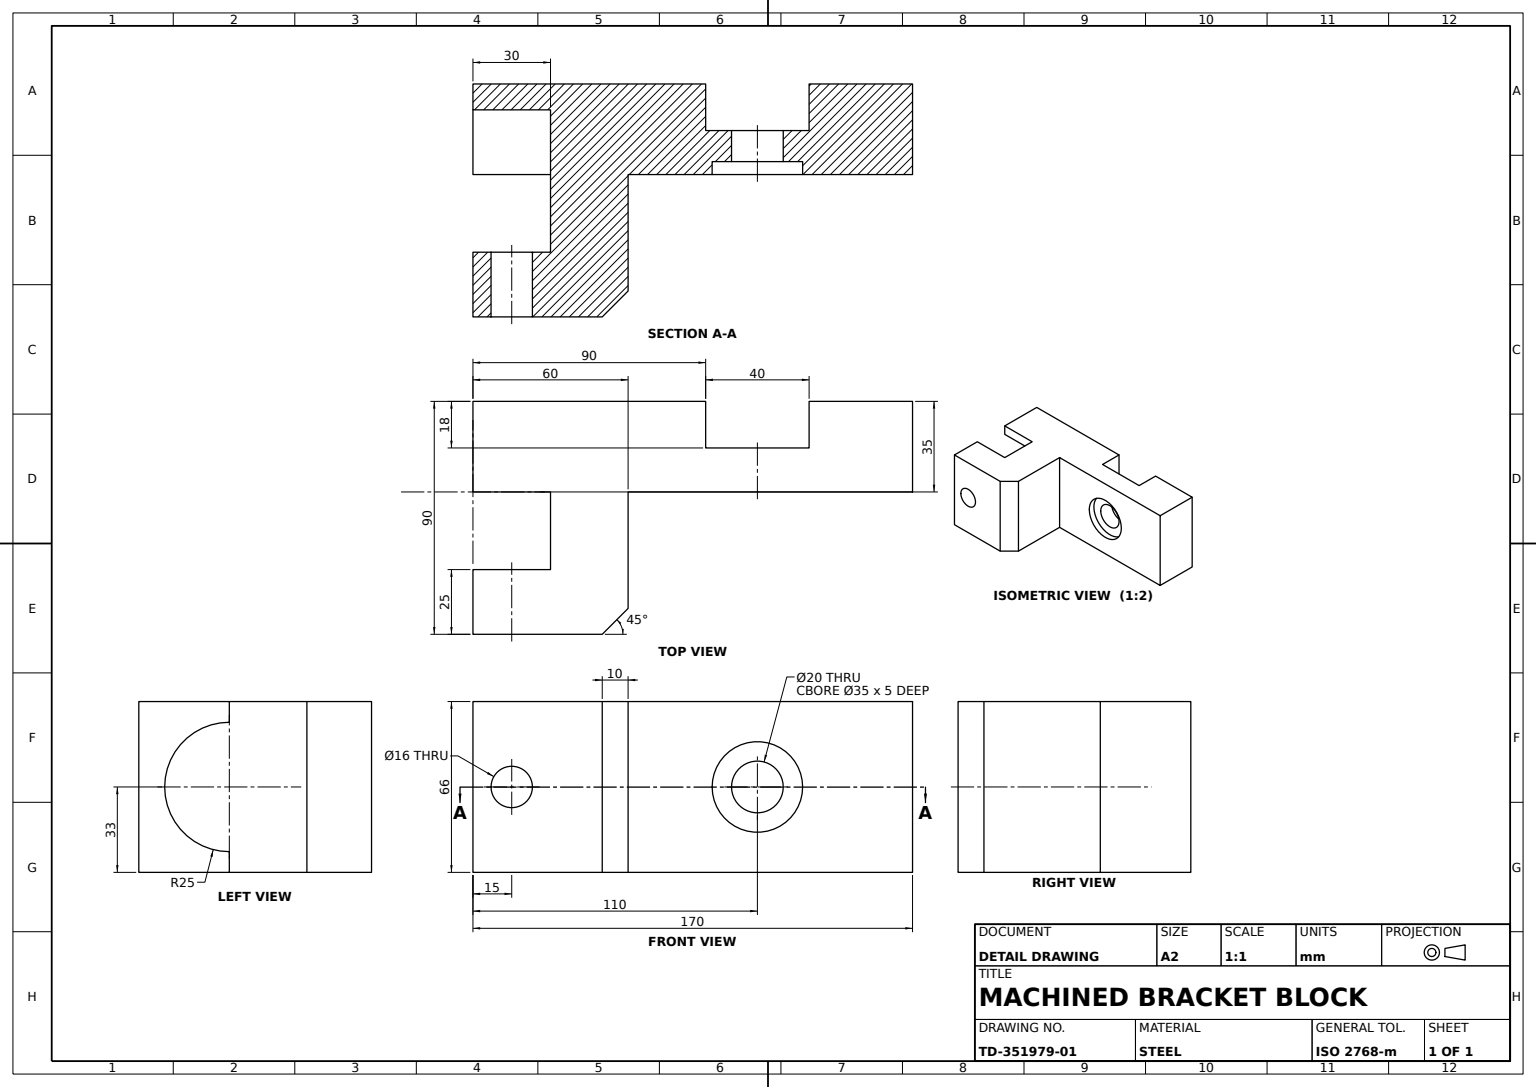
from build123d import *

# Parameters (mm, degrees)
BASE_BLOCK_PROFILE_W    = 170
BASE_BLOCK_PROFILE_H    = 66
BASE_BLOCK_DEPTH        = 35
SLOT_CUT_DEPTH          = 66
COUNTERBORE_35_SKETCH_R = 17.5
COUNTERBORE_35_DEPTH    = 5
HOLE_20_SKETCH_R        = 10
HOLE_20_DEPTH           = 12
ROUNDED_CUT_DEPTH       = 30
SIDE_LUG_DEPTH          = 66
LUG_HOLE_16_SKETCH_R    = 8
LUG_HOLE_16_DEPTH       = 66


with BuildPart() as part:
    # Base Block Profile → Base Block (new body)
    with BuildSketch(Plane.XY):
        with Locations((85, 33)):
            Rectangle(BASE_BLOCK_PROFILE_W, BASE_BLOCK_PROFILE_H)
    extrude(amount=BASE_BLOCK_DEPTH)

    # Slot Profile → Slot Cut (cut)
    with BuildSketch(Plane.XZ):
        Polygon((110, 0), (130, 0), (130, 18), (90, 18), (90, 0), align=None)
    extrude(amount=-SLOT_CUT_DEPTH, mode=Mode.SUBTRACT)

    # Counterbore Ø35 Sketch → Counterbore Ø35 (cut)
    with BuildSketch(Plane.XY.offset(35)):
        with Locations((110, 33)):
            Circle(COUNTERBORE_35_SKETCH_R)
    extrude(amount=-COUNTERBORE_35_DEPTH, mode=Mode.SUBTRACT)

    # Hole Ø20 Sketch → Hole Ø20 (cut)
    with BuildSketch(Plane.XY.offset(30)):
        with Locations((110, 33)):
            Circle(HOLE_20_SKETCH_R)
    extrude(amount=-HOLE_20_DEPTH, mode=Mode.SUBTRACT)

    # Rounded Cut Sketch → Rounded Cut (cut)
    with BuildSketch(Plane.ZY):
        with BuildLine():
            Line((35, 58), (35, 8))
            ThreePointArc((35, 8), (10, 33), (35, 58))
        make_face()
    extrude(amount=-ROUNDED_CUT_DEPTH, mode=Mode.SUBTRACT)

    # Side Lug Profile → Side Lug (add)
    with BuildSketch(Plane.XZ):
        Polygon((30, 65), (30, 35), (60, 35), (60, 80), (50, 90), (0, 90), (0, 65), align=None)
    extrude(amount=-SIDE_LUG_DEPTH)

    # Lug Hole Ø16 Sketch → Lug Hole Ø16 (cut)
    with BuildSketch(Plane.XY.offset(90)):
        with Locations((15, 33)):
            Circle(LUG_HOLE_16_SKETCH_R)
    extrude(amount=-LUG_HOLE_16_DEPTH, mode=Mode.SUBTRACT)


solid = part.part
